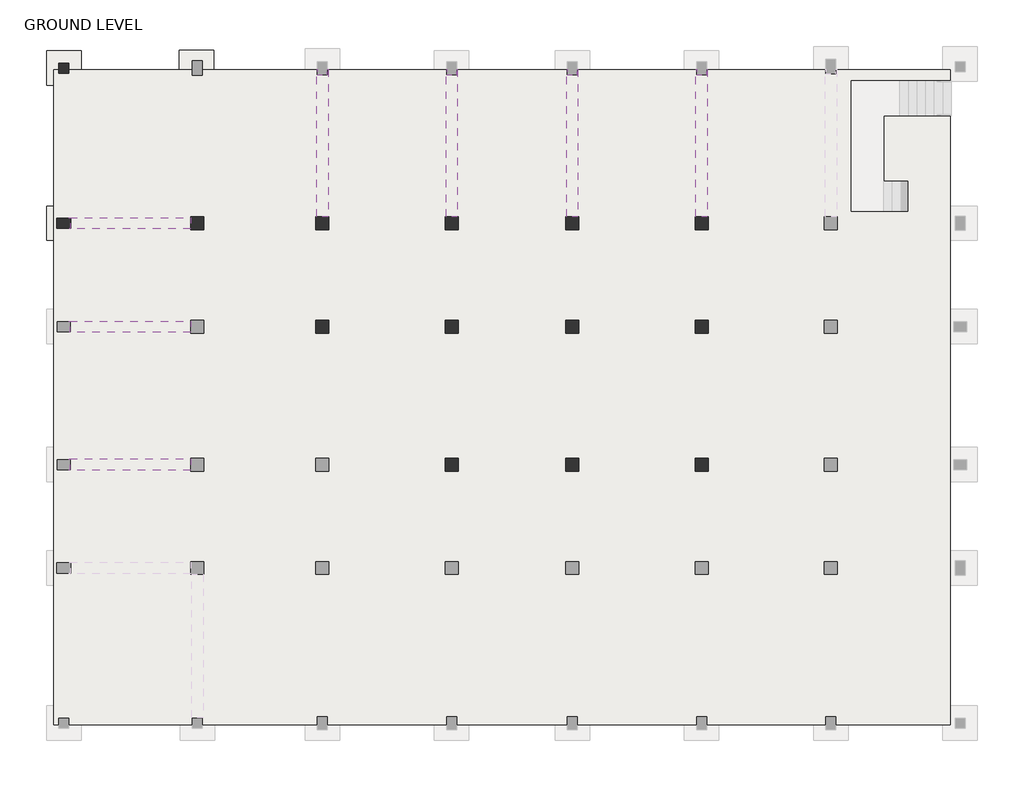
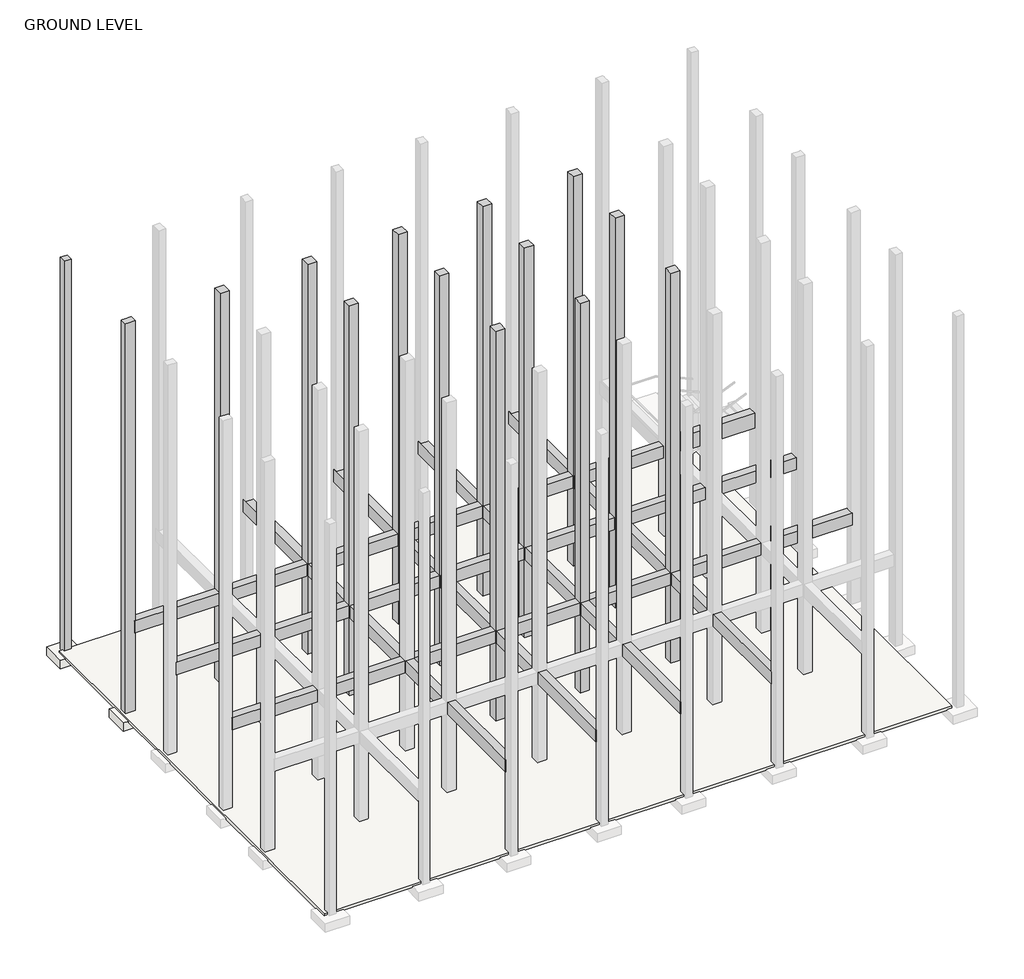
# One storey, part 2 of 3: 16 slabs, 14 columns, 7 beams.
"""IFC4 building model written with IfcOpenShell, lengths in millimetres."""

from ifc_helpers import new_model, si_unit, frame, origin, place, context, project, spatial, polyline, outline, extrude, faceted_brep, element, save

model = new_model("IFC4")

# Units and contexts
model_context = context("Model", 3, world=origin())
ifc_project = project(units=[si_unit("LENGTHUNIT", "METRE", prefix="MILLI")], contexts=[model_context])

# Site, building, storey
site = spatial("IfcSite", under=ifc_project)
building = spatial("IfcBuilding", under=site)
storey = spatial("IfcBuildingStorey", under=building, Name="GROUND LEVEL", Elevation=-1404.4011518)

# Beams
placement = place(None, origin())
element("IfcBeam", 1, ObjectType="M_Concrete-Rectangular Beam : 400 x 800mm", at=placement, inside=storey, context=model_context, shape_type="SweptSolid", body=[
    extrude(outline(polyline([(-16179.7491019, -6019.2309165), (-16535.3491019, -6019.2309165), (-16535.3491019, -6047.8309165), (-16557.5491019, -6047.8309165), (-16557.5491019, -990.0309165), (-16157.5491019, -990.0309165), (-16157.5491019, -6047.8309165), (-16179.7491019, -6047.8309165), (-16179.7491019, -6019.2309165)])), frame((0.0, 0.0, 114.4), z_axis=(0.0, 0.0, 1.0), x_axis=(1.0, 0.0, 0.0)), (0.0, 0.0, 1.0), 647.6),
    extrude(outline(polyline([(-16535.3491019, 16688.3690835), (-16179.7491019, 16688.3690835), (-16179.7491019, 16869.3690835), (-16157.5491019, 16869.3690835), (-16157.5491019, 11659.1690835), (-16557.5491019, 11659.1690835), (-16557.5491019, 16869.3690835), (-16535.3491019, 16869.3690835), (-16535.3491019, 16688.3690835)])), frame((0.0, 0.0, 114.4), z_axis=(0.0, 0.0, 1.0), x_axis=(1.0, 0.0, 0.0)), (0.0, 0.0, 1.0), 647.6),
    extrude(outline(polyline([(-16557.5491019, 11201.9690835), (-16157.5491019, 11201.9690835), (-16157.5491019, 8001.5690835), (-16557.5491019, 8001.5690835), (-16557.5491019, 11201.9690835)])), frame((0.0, 0.0, 114.4), z_axis=(0.0, 0.0, 1.0), x_axis=(1.0, 0.0, 0.0)), (0.0, 0.0, 1.0), 647.6),
    extrude(outline(polyline([(-16557.5491019, 7544.3690835), (-16157.5491019, 7544.3690835), (-16157.5491019, 3124.7690835), (-16557.5491019, 3124.7690835), (-16557.5491019, 7544.3690835)])), frame((0.0, 0.0, 114.4), z_axis=(0.0, 0.0, 1.0), x_axis=(1.0, 0.0, 0.0)), (0.0, 0.0, 1.0), 647.6),
    extrude(outline(polyline([(-16557.5491019, 2667.5690835), (-16157.5491019, 2667.5690835), (-16157.5491019, -532.8309165), (-16557.5491019, -532.8309165), (-16557.5491019, 2667.5690835)])), frame((0.0, 0.0, 114.4), z_axis=(0.0, 0.0, 1.0), x_axis=(1.0, 0.0, 0.0)), (0.0, 0.0, 1.0), 647.6),
])
element("IfcBeam", 2, ObjectType="M_Concrete-Rectangular Beam : 400 x 800mm", at=placement, inside=storey, context=model_context, shape_type="SweptSolid", body=[
    extrude(outline(polyline([(-11607.7491019, -6019.2309165), (-11963.3491019, -6019.2309165), (-11963.3491019, -6047.8309165), (-11985.5491019, -6047.8309165), (-11985.5491019, -990.0309165), (-11585.5491019, -990.0309165), (-11585.5491019, -6047.8309165), (-11607.7491019, -6047.8309165), (-11607.7491019, -6019.2309165)])), frame((0.0, 0.0, 114.4), z_axis=(0.0, 0.0, 1.0), x_axis=(1.0, 0.0, 0.0)), (0.0, 0.0, 1.0), 647.6),
    extrude(outline(polyline([(-11963.3491019, 16688.3690835), (-11607.7491019, 16688.3690835), (-11607.7491019, 16869.3690835), (-11585.5491019, 16869.3690835), (-11585.5491019, 11659.1690835), (-11985.5491019, 11659.1690835), (-11985.5491019, 16869.3690835), (-11963.3491019, 16869.3690835), (-11963.3491019, 16688.3690835)])), frame((0.0, 0.0, 114.4), z_axis=(0.0, 0.0, 1.0), x_axis=(1.0, 0.0, 0.0)), (0.0, 0.0, 1.0), 647.6),
    extrude(outline(polyline([(-11985.5491019, 11201.9690835), (-11585.5491019, 11201.9690835), (-11585.5491019, 8001.5690835), (-11985.5491019, 8001.5690835), (-11985.5491019, 11201.9690835)])), frame((0.0, 0.0, 114.4), z_axis=(0.0, 0.0, 1.0), x_axis=(1.0, 0.0, 0.0)), (0.0, 0.0, 1.0), 647.6),
    extrude(outline(polyline([(-11985.5491019, 7544.3690835), (-11585.5491019, 7544.3690835), (-11585.5491019, 3124.7690835), (-11985.5491019, 3124.7690835), (-11985.5491019, 7544.3690835)])), frame((0.0, 0.0, 114.4), z_axis=(0.0, 0.0, 1.0), x_axis=(1.0, 0.0, 0.0)), (0.0, 0.0, 1.0), 647.6),
    extrude(outline(polyline([(-11585.5491019, -532.8309165), (-11985.5491019, -532.8309165), (-11985.5491019, 2667.5690835), (-11585.5491019, 2667.5690835), (-11585.5491019, -532.8309165)])), frame((0.0, 0.0, 114.4), z_axis=(0.0, 0.0, 1.0), x_axis=(1.0, 0.0, 0.0)), (0.0, 0.0, 1.0), 647.6),
])
element("IfcBeam", 3, ObjectType="M_Concrete-Rectangular Beam : 400 x 800mm", at=placement, inside=storey, context=model_context, shape_type="SweptSolid", body=[
    extrude(outline(polyline([(-7340.5491019, -6019.2309165), (-7696.1491019, -6019.2309165), (-7696.1491019, -6047.8309165), (-7718.3491019, -6047.8309165), (-7718.3491019, -990.0309165), (-7318.3491019, -990.0309165), (-7318.3491019, -6047.8309165), (-7340.5491019, -6047.8309165), (-7340.5491019, -6019.2309165)])), frame((0.0, 0.0, 114.4), z_axis=(0.0, 0.0, 1.0), x_axis=(1.0, 0.0, 0.0)), (0.0, 0.0, 1.0), 647.6),
    extrude(outline(polyline([(-7696.1491019, 16688.3690835), (-7340.5491019, 16688.3690835), (-7340.5491019, 16869.3690835), (-7318.3491019, 16869.3690835), (-7318.3491019, 11659.1690835), (-7718.3491019, 11659.1690835), (-7718.3491019, 16869.3690835), (-7696.1491019, 16869.3690835), (-7696.1491019, 16688.3690835)])), frame((0.0, 0.0, 114.4), z_axis=(0.0, 0.0, 1.0), x_axis=(1.0, 0.0, 0.0)), (0.0, 0.0, 1.0), 647.6),
    extrude(outline(polyline([(-7718.3491019, 7544.3690835), (-7318.3491019, 7544.3690835), (-7318.3491019, 3124.7690835), (-7718.3491019, 3124.7690835), (-7718.3491019, 7544.3690835)])), frame((0.0, 0.0, 114.4), z_axis=(0.0, 0.0, 1.0), x_axis=(1.0, 0.0, 0.0)), (0.0, 0.0, 1.0), 647.6),
    extrude(outline(polyline([(-7318.3491019, 8001.5690835), (-7718.3491019, 8001.5690835), (-7718.3491019, 11201.9690835), (-7318.3491019, 11201.9690835), (-7318.3491019, 8001.5690835)])), frame((0.0, 0.0, 114.4), z_axis=(0.0, 0.0, 1.0), x_axis=(1.0, 0.0, 0.0)), (0.0, 0.0, 1.0), 647.6),
    extrude(outline(polyline([(-7318.3491019, -532.8309165), (-7718.3491019, -532.8309165), (-7718.3491019, 2667.5690835), (-7318.3491019, 2667.5690835), (-7318.3491019, -532.8309165)])), frame((0.0, 0.0, 114.4), z_axis=(0.0, 0.0, 1.0), x_axis=(1.0, 0.0, 0.0)), (0.0, 0.0, 1.0), 647.6),
])
element("IfcBeam", 4, ObjectType="M_Concrete-Rectangular Beam : 400 x 800mm", at=placement, inside=storey, context=model_context, shape_type="SweptSolid", body=[
    extrude(outline(polyline([(-2768.5491019, -6019.2309165), (-3124.1491019, -6019.2309165), (-3124.1491019, -6047.8309165), (-3146.3491019, -6047.8309165), (-3146.3491019, -990.0309165), (-2746.3491019, -990.0309165), (-2746.3491019, -6047.8309165), (-2768.5491019, -6047.8309165), (-2768.5491019, -6019.2309165)])), frame((0.0, 0.0, 114.4), z_axis=(0.0, 0.0, 1.0), x_axis=(1.0, 0.0, 0.0)), (0.0, 0.0, 1.0), 647.6),
    extrude(outline(polyline([(-3124.1491019, 16688.3690835), (-2768.5491019, 16688.3690835), (-2768.5491019, 16869.3690835), (-2746.3491019, 16869.3690835), (-2746.3491019, 11659.1690835), (-3146.3491019, 11659.1690835), (-3146.3491019, 16869.3690835), (-3124.1491019, 16869.3690835), (-3124.1491019, 16688.3690835)])), frame((0.0, 0.0, 114.4), z_axis=(0.0, 0.0, 1.0), x_axis=(1.0, 0.0, 0.0)), (0.0, 0.0, 1.0), 647.6),
    extrude(outline(polyline([(-3146.3491019, 11201.9690835), (-2746.3491019, 11201.9690835), (-2746.3491019, 8001.5690835), (-3146.3491019, 8001.5690835), (-3146.3491019, 11201.9690835)])), frame((0.0, 0.0, 114.4), z_axis=(0.0, 0.0, 1.0), x_axis=(1.0, 0.0, 0.0)), (0.0, 0.0, 1.0), 647.6),
    extrude(outline(polyline([(-3146.3491019, 7544.3690835), (-2746.3491019, 7544.3690835), (-2746.3491019, 3124.7690835), (-3146.3491019, 3124.7690835), (-3146.3491019, 7544.3690835)])), frame((0.0, 0.0, 114.4), z_axis=(0.0, 0.0, 1.0), x_axis=(1.0, 0.0, 0.0)), (0.0, 0.0, 1.0), 647.6),
    extrude(outline(polyline([(-2746.3491019, -532.8309165), (-3146.3491019, -532.8309165), (-3146.3491019, 2667.5690835), (-2746.3491019, 2667.5690835), (-2746.3491019, -532.8309165)])), frame((0.0, 0.0, 114.4), z_axis=(0.0, 0.0, 1.0), x_axis=(1.0, 0.0, 0.0)), (0.0, 0.0, 1.0), 647.6),
])
element("IfcBeam", 5, ObjectType="M_Concrete-Rectangular Beam : 400 x 800mm", at=placement, inside=storey, context=model_context, shape_type="SweptSolid", body=[
    extrude(outline(polyline([(-25247.5491019, 11252.7690835), (-25247.5491019, 11608.3690835), (-25301.5491019, 11608.3690835), (-25301.5491019, 11630.5690835), (-21005.7491019, 11630.5690835), (-21005.7491019, 11230.5690835), (-25301.5491019, 11230.5690835), (-25301.5491019, 11252.7690835), (-25247.5491019, 11252.7690835)])), frame((0.0, 0.0, 114.4), z_axis=(0.0, 0.0, 1.0), x_axis=(1.0, 0.0, 0.0)), (0.0, 0.0, 1.0), 647.6),
    extrude(outline(polyline([(-20548.5491019, 11230.5690835), (-20548.5491019, 11630.5690835), (-16586.1491019, 11630.5690835), (-16586.1491019, 11230.5690835), (-20548.5491019, 11230.5690835)])), frame((0.0, 0.0, 114.4), z_axis=(0.0, 0.0, 1.0), x_axis=(1.0, 0.0, 0.0)), (0.0, 0.0, 1.0), 647.6),
    extrude(outline(polyline([(-16128.9491019, 11230.5690835), (-16128.9491019, 11630.5690835), (-12014.1491019, 11630.5690835), (-12014.1491019, 11230.5690835), (-16128.9491019, 11230.5690835)])), frame((0.0, 0.0, 114.4), z_axis=(0.0, 0.0, 1.0), x_axis=(1.0, 0.0, 0.0)), (0.0, 0.0, 1.0), 647.6),
    extrude(outline(polyline([(-11556.9491019, 11230.5690835), (-11556.9491019, 11630.5690835), (-7746.9491019, 11630.5690835), (-7746.9491019, 11230.5690835), (-11556.9491019, 11230.5690835)])), frame((0.0, 0.0, 114.4), z_axis=(0.0, 0.0, 1.0), x_axis=(1.0, 0.0, 0.0)), (0.0, 0.0, 1.0), 647.6),
    extrude(outline(polyline([(-7289.7491019, 11230.5690835), (-7289.7491019, 11630.5690835), (-3174.9491019, 11630.5690835), (-3174.9491019, 11230.5690835), (-7289.7491019, 11230.5690835)])), frame((0.0, 0.0, 114.4), z_axis=(0.0, 0.0, 1.0), x_axis=(1.0, 0.0, 0.0)), (0.0, 0.0, 1.0), 647.6),
    extrude(outline(polyline([(-2717.7491019, 11230.5690835), (-2717.7491019, 11630.5690835), (1397.0508981, 11630.5690835), (1397.0508981, 11230.5690835), (-2717.7491019, 11230.5690835)])), frame((0.0, 0.0, 114.4), z_axis=(0.0, 0.0, 1.0), x_axis=(1.0, 0.0, 0.0)), (0.0, 0.0, 1.0), 647.6),
    extrude(outline(polyline([(1854.2508981, 11230.5690835), (1854.2508981, 11630.5690835), (5997.6508981, 11630.5690835), (5997.6508981, 11230.5690835), (1854.2508981, 11230.5690835)])), frame((0.0, 0.0, 114.4), z_axis=(0.0, 0.0, 1.0), x_axis=(1.0, 0.0, 0.0)), (0.0, 0.0, 1.0), 800.0),
])
element("IfcBeam", 6, ObjectType="M_Concrete-Rectangular Beam : 400 x 800mm", at=placement, inside=storey, context=model_context, shape_type="SweptSolid", body=[
    extrude(outline(polyline([(-25272.9491019, 2718.3690835), (-25272.9491019, 3073.9690835), (-25301.5491019, 3073.9690835), (-25301.5491019, 3096.1690835), (-21005.7491019, 3096.1690835), (-21005.7491019, 2696.1690835), (-25301.5491019, 2696.1690835), (-25301.5491019, 2718.3690835), (-25272.9491019, 2718.3690835)])), frame((0.0, 0.0, 114.4), z_axis=(0.0, 0.0, 1.0), x_axis=(1.0, 0.0, 0.0)), (0.0, 0.0, 1.0), 647.6),
    extrude(outline(polyline([(5969.0508981, 3073.9690835), (5969.0508981, 2718.3690835), (5997.6508981, 2718.3690835), (5997.6508981, 2696.1690835), (1854.2508981, 2696.1690835), (1854.2508981, 3096.1690835), (5997.6508981, 3096.1690835), (5997.6508981, 3073.9690835), (5969.0508981, 3073.9690835)])), frame((0.0, 0.0, 114.4), z_axis=(0.0, 0.0, 1.0), x_axis=(1.0, 0.0, 0.0)), (0.0, 0.0, 1.0), 647.6),
    extrude(outline(polyline([(-20548.5491019, 2696.1690835), (-20548.5491019, 3096.1690835), (-16586.1491019, 3096.1690835), (-16586.1491019, 2696.1690835), (-20548.5491019, 2696.1690835)])), frame((0.0, 0.0, 114.4), z_axis=(0.0, 0.0, 1.0), x_axis=(1.0, 0.0, 0.0)), (0.0, 0.0, 1.0), 647.6),
    extrude(outline(polyline([(-16128.9491019, 2696.1690835), (-16128.9491019, 3096.1690835), (-12014.1491019, 3096.1690835), (-12014.1491019, 2696.1690835), (-16128.9491019, 2696.1690835)])), frame((0.0, 0.0, 114.4), z_axis=(0.0, 0.0, 1.0), x_axis=(1.0, 0.0, 0.0)), (0.0, 0.0, 1.0), 647.6),
    extrude(outline(polyline([(1397.0508981, 3096.1690835), (1397.0508981, 2696.1690835), (-2717.7491019, 2696.1690835), (-2717.7491019, 3096.1690835), (1397.0508981, 3096.1690835)])), frame((0.0, 0.0, 114.4), z_axis=(0.0, 0.0, 1.0), x_axis=(1.0, 0.0, 0.0)), (0.0, 0.0, 1.0), 647.6),
    extrude(outline(polyline([(-3174.9491019, 3096.1690835), (-3174.9491019, 2696.1690835), (-7289.7491019, 2696.1690835), (-7289.7491019, 3096.1690835), (-3174.9491019, 3096.1690835)])), frame((0.0, 0.0, 114.4), z_axis=(0.0, 0.0, 1.0), x_axis=(1.0, 0.0, 0.0)), (0.0, 0.0, 1.0), 647.6),
    extrude(outline(polyline([(-7746.9491019, 3096.1690835), (-7746.9491019, 2696.1690835), (-11556.9491019, 2696.1690835), (-11556.9491019, 3096.1690835), (-7746.9491019, 3096.1690835)])), frame((0.0, 0.0, 114.4), z_axis=(0.0, 0.0, 1.0), x_axis=(1.0, 0.0, 0.0)), (0.0, 0.0, 1.0), 647.6),
])
element("IfcBeam", 7, ObjectType="M_Concrete-Rectangular Beam : 400 x 800mm", at=placement, inside=storey, context=model_context, shape_type="SweptSolid", body=[
    extrude(outline(polyline([(-25272.9491019, 7595.1690835), (-25272.9491019, 7950.7690835), (-25301.5491019, 7950.7690835), (-25301.5491019, 7972.9690835), (-21005.7491019, 7972.9690835), (-21005.7491019, 7572.9690835), (-25301.5491019, 7572.9690835), (-25301.5491019, 7595.1690835), (-25272.9491019, 7595.1690835)])), frame((0.0, 0.0, 114.4), z_axis=(0.0, 0.0, 1.0), x_axis=(1.0, 0.0, 0.0)), (0.0, 0.0, 1.0), 647.6),
    extrude(outline(polyline([(5969.0508981, 7950.7690835), (5969.0508981, 7595.1690835), (5997.6508981, 7595.1690835), (5997.6508981, 7572.9690835), (1854.2508981, 7572.9690835), (1854.2508981, 7972.9690835), (5997.6508981, 7972.9690835), (5997.6508981, 7950.7690835), (5969.0508981, 7950.7690835)])), frame((0.0, 0.0, 114.4), z_axis=(0.0, 0.0, 1.0), x_axis=(1.0, 0.0, 0.0)), (0.0, 0.0, 1.0), 647.6),
    extrude(outline(polyline([(-7289.7491019, 7572.9690835), (-7289.7491019, 7972.9690835), (-3174.9491019, 7972.9690835), (-3174.9491019, 7572.9690835), (-7289.7491019, 7572.9690835)])), frame((0.0, 0.0, 114.4), z_axis=(0.0, 0.0, 1.0), x_axis=(1.0, 0.0, 0.0)), (0.0, 0.0, 1.0), 647.6),
    extrude(outline(polyline([(-7746.9491019, 7972.9690835), (-7746.9491019, 7572.9690835), (-11556.9491019, 7572.9690835), (-11556.9491019, 7972.9690835), (-7746.9491019, 7972.9690835)])), frame((0.0, 0.0, 114.4), z_axis=(0.0, 0.0, 1.0), x_axis=(1.0, 0.0, 0.0)), (0.0, 0.0, 1.0), 647.6),
    extrude(outline(polyline([(1397.0508981, 7972.9690835), (1397.0508981, 7572.9690835), (-2717.7491019, 7572.9690835), (-2717.7491019, 7972.9690835), (1397.0508981, 7972.9690835)])), frame((0.0, 0.0, 114.4), z_axis=(0.0, 0.0, 1.0), x_axis=(1.0, 0.0, 0.0)), (0.0, 0.0, 1.0), 647.6),
    extrude(outline(polyline([(-12014.1491019, 7972.9690835), (-12014.1491019, 7572.9690835), (-16128.9491019, 7572.9690835), (-16128.9491019, 7972.9690835), (-12014.1491019, 7972.9690835)])), frame((0.0, 0.0, 114.4), z_axis=(0.0, 0.0, 1.0), x_axis=(1.0, 0.0, 0.0)), (0.0, 0.0, 1.0), 647.6),
    extrude(outline(polyline([(-16586.1491019, 7972.9690835), (-16586.1491019, 7572.9690835), (-20548.5491019, 7572.9690835), (-20548.5491019, 7972.9690835), (-16586.1491019, 7972.9690835)])), frame((0.0, 0.0, 114.4), z_axis=(0.0, 0.0, 1.0), x_axis=(1.0, 0.0, 0.0)), (0.0, 0.0, 1.0), 647.6),
])

# Columns
element("IfcColumn", 8, ObjectType="M_Concrete-Rectangular-Column : C1", at=placement, inside=storey, context=model_context, shape_type="SweptSolid", body=[
    extrude(outline(polyline([(-25323.7491019, 17094.7690835), (-25323.7491019, 16739.1690835), (-25679.3491019, 16739.1690835), (-25679.3491019, 17094.7690835), (-25323.7491019, 17094.7690835)])), frame((0.0, 0.0, -4147.6011518), z_axis=(0.0, 0.0, 1.0), x_axis=(1.0, 0.0, 0.0)), (0.0, 0.0, 1.0), 20911.6011518),
])
element("IfcColumn", 9, ObjectType="M_Concrete-Rectangular-Column : C3", at=placement, inside=storey, context=model_context, shape_type="SweptSolid", body=[
    extrude(outline(polyline([(-7289.7491019, 8001.5690835), (-7289.7491019, 7544.3690835), (-7746.9491019, 7544.3690835), (-7746.9491019, 8001.5690835), (-7289.7491019, 8001.5690835)])), frame((0.0, 0.0, -4147.6011518), z_axis=(0.0, 0.0, 1.0), x_axis=(1.0, 0.0, 0.0)), (0.0, 0.0, 1.0), 20911.6011518),
])
element("IfcColumn", 10, ObjectType="M_Concrete-Rectangular-Column : C3", at=placement, inside=storey, context=model_context, shape_type="SweptSolid", body=[
    extrude(outline(polyline([(-20548.5491019, 11659.1690835), (-20548.5491019, 11201.9690835), (-21005.7491019, 11201.9690835), (-21005.7491019, 11659.1690835), (-20548.5491019, 11659.1690835)])), frame((0.0, 0.0, -4147.6011518), z_axis=(0.0, 0.0, 1.0), x_axis=(1.0, 0.0, 0.0)), (0.0, 0.0, 1.0), 20911.6011518),
])
element("IfcColumn", 11, ObjectType="M_Concrete-Rectangular-Column : C3", at=placement, inside=storey, context=model_context, shape_type="SweptSolid", body=[
    extrude(outline(polyline([(-16128.9491019, 11659.1690835), (-16128.9491019, 11201.9690835), (-16586.1491019, 11201.9690835), (-16586.1491019, 11659.1690835), (-16128.9491019, 11659.1690835)])), frame((0.0, 0.0, -4147.6011518), z_axis=(0.0, 0.0, 1.0), x_axis=(1.0, 0.0, 0.0)), (0.0, 0.0, 1.0), 20911.6011518),
])
element("IfcColumn", 12, ObjectType="M_Concrete-Rectangular-Column : C3", at=placement, inside=storey, context=model_context, shape_type="SweptSolid", body=[
    extrude(outline(polyline([(-11556.9491019, 11659.1690835), (-11556.9491019, 11201.9690835), (-12014.1491019, 11201.9690835), (-12014.1491019, 11659.1690835), (-11556.9491019, 11659.1690835)])), frame((0.0, 0.0, -4147.6011518), z_axis=(0.0, 0.0, 1.0), x_axis=(1.0, 0.0, 0.0)), (0.0, 0.0, 1.0), 20911.6011518),
])
element("IfcColumn", 13, ObjectType="M_Concrete-Rectangular-Column : C3", at=placement, inside=storey, context=model_context, shape_type="SweptSolid", body=[
    extrude(outline(polyline([(-7289.7491019, 11659.1690835), (-7289.7491019, 11201.9690835), (-7746.9491019, 11201.9690835), (-7746.9491019, 11659.1690835), (-7289.7491019, 11659.1690835)])), frame((0.0, 0.0, -4147.6011518), z_axis=(0.0, 0.0, 1.0), x_axis=(1.0, 0.0, 0.0)), (0.0, 0.0, 1.0), 20911.6011518),
])
element("IfcColumn", 14, ObjectType="M_Concrete-Rectangular-Column : C3", at=placement, inside=storey, context=model_context, shape_type="SweptSolid", body=[
    extrude(outline(polyline([(-2717.7491019, 11659.1690835), (-2717.7491019, 11201.9690835), (-3174.9491019, 11201.9690835), (-3174.9491019, 11659.1690835), (-2717.7491019, 11659.1690835)])), frame((0.0, 0.0, -4147.6011518), z_axis=(0.0, 0.0, 1.0), x_axis=(1.0, 0.0, 0.0)), (0.0, 0.0, 1.0), 20911.6011518),
])
element("IfcColumn", 15, ObjectType="M_Concrete-Rectangular-Column : C3", at=placement, inside=storey, context=model_context, shape_type="SweptSolid", body=[
    extrude(outline(polyline([(-2717.7491019, 8001.5690835), (-2717.7491019, 7544.3690835), (-3174.9491019, 7544.3690835), (-3174.9491019, 8001.5690835), (-2717.7491019, 8001.5690835)])), frame((0.0, 0.0, -4147.6011518), z_axis=(0.0, 0.0, 1.0), x_axis=(1.0, 0.0, 0.0)), (0.0, 0.0, 1.0), 20911.6011518),
])
element("IfcColumn", 16, ObjectType="M_Concrete-Rectangular-Column : C3", at=placement, inside=storey, context=model_context, shape_type="SweptSolid", body=[
    extrude(outline(polyline([(-11556.9491019, 8001.5690835), (-11556.9491019, 7544.3690835), (-12014.1491019, 7544.3690835), (-12014.1491019, 8001.5690835), (-11556.9491019, 8001.5690835)])), frame((0.0, 0.0, -4147.6011518), z_axis=(0.0, 0.0, 1.0), x_axis=(1.0, 0.0, 0.0)), (0.0, 0.0, 1.0), 20911.6011518),
])
element("IfcColumn", 17, ObjectType="M_Concrete-Rectangular-Column : C3", at=placement, inside=storey, context=model_context, shape_type="SweptSolid", body=[
    extrude(outline(polyline([(-16128.9491019, 8001.5690835), (-16128.9491019, 7544.3690835), (-16586.1491019, 7544.3690835), (-16586.1491019, 8001.5690835), (-16128.9491019, 8001.5690835)])), frame((0.0, 0.0, -4147.6011518), z_axis=(0.0, 0.0, 1.0), x_axis=(1.0, 0.0, 0.0)), (0.0, 0.0, 1.0), 20911.6011518),
])
element("IfcColumn", 18, ObjectType="M_Concrete-Rectangular-Column : C3", at=placement, inside=storey, context=model_context, shape_type="SweptSolid", body=[
    extrude(outline(polyline([(-2717.7491019, 3124.7690835), (-2717.7491019, 2667.5690835), (-3174.9491019, 2667.5690835), (-3174.9491019, 3124.7690835), (-2717.7491019, 3124.7690835)])), frame((0.0, 0.0, -4147.6011518), z_axis=(0.0, 0.0, 1.0), x_axis=(1.0, 0.0, 0.0)), (0.0, 0.0, 1.0), 20911.6011518),
])
element("IfcColumn", 19, ObjectType="M_Concrete-Rectangular-Column : C3", at=placement, inside=storey, context=model_context, shape_type="SweptSolid", body=[
    extrude(outline(polyline([(-7289.7491019, 3124.7690835), (-7289.7491019, 2667.5690835), (-7746.9491019, 2667.5690835), (-7746.9491019, 3124.7690835), (-7289.7491019, 3124.7690835)])), frame((0.0, 0.0, -4147.6011518), z_axis=(0.0, 0.0, 1.0), x_axis=(1.0, 0.0, 0.0)), (0.0, 0.0, 1.0), 20911.6011518),
])
element("IfcColumn", 20, ObjectType="M_Concrete-Rectangular-Column : C3", at=placement, inside=storey, context=model_context, shape_type="SweptSolid", body=[
    extrude(outline(polyline([(-11556.9491019, 3124.7690835), (-11556.9491019, 2667.5690835), (-12014.1491019, 2667.5690835), (-12014.1491019, 3124.7690835), (-11556.9491019, 3124.7690835)])), frame((0.0, 0.0, -4147.6011518), z_axis=(0.0, 0.0, 1.0), x_axis=(1.0, 0.0, 0.0)), (0.0, 0.0, 1.0), 20911.6011518),
])
element("IfcColumn", 21, ObjectType="M_Concrete-Rectangular-Column : C4", at=placement, inside=storey, context=model_context, shape_type="Brep", body=[
    faceted_brep([(-25755.5491019, 11608.3690835, -4147.6011518), (-25247.5491019, 11608.3690835, -4147.6011518), (-25247.5491019, 11252.7690835, -4147.6011518), (-25755.5491019, 11252.7690835, -4147.6011518), (-25755.5491019, 11608.3690835, 16764.0), (-25701.5491019, 11608.3690835, 16764.0), (-25679.3491019, 11608.3690835, 16764.0), (-25247.5491019, 11608.3690835, 16764.0), (-25247.5491019, 11252.7690835, 16764.0), (-25679.3491019, 11252.7690835, 16764.0), (-25701.5491019, 11252.7690835, 16764.0), (-25755.5491019, 11252.7690835, 16764.0)], [[[0, 1, 2, 3]], [[4, 5, 6, 7, 1, 0]], [[7, 8, 2, 1]], [[8, 9, 10, 11, 3, 2]], [[11, 4, 0, 3]], [[4, 11, 10, 9, 8, 7, 6, 5]]]),
])

# Slabs
element("IfcSlab", 22, ObjectType="6\" Foundation Slab", at=placement, inside=storey, context=model_context, shape_type="Brep", body=[
    faceted_brep([(5842.0508981, 16861.9544764, -4197.8282159), (5842.0508981, 16459.7690835, -4197.8282159), (5842.0508981, 12040.1690835, -4197.8282159), (5842.0508981, 10820.9690835, -4197.8282159), (5842.0508981, 8382.5690835, -4197.8282159), (5842.0508981, 7163.3690835, -4197.8282159), (5842.0508981, 3505.7690835, -4197.8282159), (5842.0508981, 2286.5690835, -4197.8282159), (5842.0508981, -151.8309165, -4197.8282159), (5842.0508981, -1371.0309165, -4197.8282159), (5842.0508981, -5638.2309165, -4197.8282159), (5842.0508981, -6302.8455236, -4197.8282159), (5588.0508981, -6302.8455236, -4197.8282159), (2235.2508981, -6302.8455236, -4197.8282159), (1016.0508981, -6302.8455236, -4197.8282159), (-2336.7491019, -6302.8455236, -4197.8282159), (-3555.9491019, -6302.8455236, -4197.8282159), (-6908.7491019, -6302.8455236, -4197.8282159), (-8127.9491019, -6302.8455236, -4197.8282159), (-11175.9491019, -6302.8455236, -4197.8282159), (-12395.1491019, -6302.8455236, -4197.8282159), (-15747.9491019, -6302.8455236, -4197.8282159), (-16967.1491019, -6302.8455236, -4197.8282159), (-20167.5491019, -6302.8455236, -4197.8282159), (-21386.7491019, -6302.8455236, -4197.8282159), (-24891.9491019, -6302.8455236, -4197.8282159), (-25857.1491019, -6302.8455236, -4197.8282159), (-25857.1491019, -5638.2309165, -4197.8282159), (-25857.1491019, -1371.0309165, -4197.8282159), (-25857.1491019, -151.8309165, -4197.8282159), (-25857.1491019, 2286.5690835, -4197.8282159), (-25857.1491019, 3505.7690835, -4197.8282159), (-25857.1491019, 7163.3690835, -4197.8282159), (-25857.1491019, 8382.5690835, -4197.8282159), (-25857.1491019, 10820.9690835, -4197.8282159), (-25857.1491019, 12040.1690835, -4197.8282159), (-25857.1491019, 16307.3690835, -4197.8282159), (-25857.1491019, 16861.9544764, -4197.8282159), (-24891.9491019, 16861.9544764, -4197.8282159), (-21412.1491019, 16861.9544764, -4197.8282159), (-20192.9491019, 16861.9544764, -4197.8282159), (-16967.1491019, 16861.9544764, -4197.8282159), (-15747.9491019, 16861.9544764, -4197.8282159), (-12395.1491019, 16861.9544764, -4197.8282159), (-11175.9491019, 16861.9544764, -4197.8282159), (-8127.9491019, 16861.9544764, -4197.8282159), (-6908.7491019, 16861.9544764, -4197.8282159), (-3555.9491019, 16861.9544764, -4197.8282159), (-2336.7491019, 16861.9544764, -4197.8282159), (1016.0508981, 16861.9544764, -4197.8282159), (2235.2508981, 16861.9544764, -4197.8282159), (5588.0508981, 16861.9544764, -4197.8282159), (5842.0508981, 16861.9544764, -4045.4282159), (-25857.1491019, 16861.9544764, -4045.4282159), (-25857.1491019, -6302.8455236, -4045.4282159), (5842.0508981, -6302.8455236, -4045.4282159), (5842.0508981, 16861.9544764, -4147.6011518), (5842.0508981, -6302.8455236, -4147.6011518), (-25857.1491019, -6302.8455236, -4147.6011518), (-25857.1491019, 16861.9544764, -4147.6011518)], [[[0, 1, 2, 3, 4, 5, 6, 7, 8, 9, 10, 11, 12, 13, 14, 15, 16, 17, 18, 19, 20, 21, 22, 23, 24, 25, 26, 27, 28, 29, 30, 31, 32, 33, 34, 35, 36, 37, 38, 39, 40, 41, 42, 43, 44, 45, 46, 47, 48, 49, 50, 51]], [[52, 53, 54, 55]], [[11, 10, 9, 8, 7, 6, 5, 4, 3, 2, 1, 0, 56, 52, 55, 57]], [[26, 25, 24, 23, 22, 21, 20, 19, 18, 17, 16, 15, 14, 13, 12, 11, 57, 55, 54, 58]], [[37, 36, 35, 34, 33, 32, 31, 30, 29, 28, 27, 26, 58, 54, 53, 59]], [[0, 51, 50, 49, 48, 47, 46, 45, 44, 43, 42, 41, 40, 39, 38, 37, 59, 53, 52, 56]]]),
])
element("IfcSlab", 23, ObjectType="M_Footing-Rectangular : F 5", at=placement, inside=storey, context=model_context, shape_type="Brep", body=[
    faceted_brep([(-24891.9491019, 17526.5690835, -4147.6011518), (-26111.1491019, 17526.5690835, -4147.6011518), (-26111.1491019, 16307.3690835, -4147.6011518), (-25857.1491019, 16307.3690835, -4147.6011518), (-25857.1491019, 16861.9544764, -4147.6011518), (-24891.9491019, 16861.9544764, -4147.6011518), (-24891.9491019, 17526.5690835, -4597.6011518), (-24891.9491019, 16307.3690835, -4597.6011518), (-26111.1491019, 16307.3690835, -4597.6011518), (-26111.1491019, 17526.5690835, -4597.6011518), (-24891.9491019, 16307.3690835, -4197.8282159), (-25857.1491019, 16307.3690835, -4197.8282159), (-24891.9491019, 16861.9544764, -4197.8282159), (-25857.1491019, 16861.9544764, -4197.8282159)], [[[0, 1, 2, 3, 4, 5]], [[6, 7, 8, 9]], [[1, 0, 6, 9]], [[2, 1, 9, 8]], [[8, 7, 10, 11, 3, 2]], [[7, 6, 0, 5, 12, 10]], [[12, 13, 11, 10]], [[13, 12, 5, 4]], [[11, 13, 4, 3]]]),
])
element("IfcSlab", 24, ObjectType="M_Footing-Rectangular : F 5", at=placement, inside=storey, context=model_context, shape_type="SweptSolid", body=[
    extrude(outline(polyline([(17551.9690835, -4597.6011518), (16332.7690835, -4597.6011518), (16332.7690835, -4197.8282159), (16861.9544764, -4197.8282159), (16861.9544764, -4147.6011518), (17551.9690835, -4147.6011518), (17551.9690835, -4597.6011518)])), frame((-21412.1491019, 0.0, 0.0), z_axis=(1.0, 0.0, 0.0), x_axis=(0.0, 1.0, 0.0)), (0.0, 0.0, 1.0), 1219.2),
])
element("IfcSlab", 25, ObjectType="M_Footing-Rectangular : F 5", at=placement, inside=storey, context=model_context, shape_type="SweptSolid", body=[
    extrude(outline(polyline([(-2336.7491019, 12040.1690835), (-2336.7491019, 10820.9690835), (-3555.9491019, 10820.9690835), (-3555.9491019, 12040.1690835), (-2336.7491019, 12040.1690835)])), frame((0.0, 0.0, -4597.6011518), z_axis=(0.0, 0.0, 1.0), x_axis=(1.0, 0.0, 0.0)), (0.0, 0.0, 1.0), 399.772936),
])
element("IfcSlab", 26, ObjectType="M_Footing-Rectangular : F 5", at=placement, inside=storey, context=model_context, shape_type="SweptSolid", body=[
    extrude(outline(polyline([(-6908.7491019, 12040.1690835), (-6908.7491019, 10820.9690835), (-8127.9491019, 10820.9690835), (-8127.9491019, 12040.1690835), (-6908.7491019, 12040.1690835)])), frame((0.0, 0.0, -4597.6011518), z_axis=(0.0, 0.0, 1.0), x_axis=(1.0, 0.0, 0.0)), (0.0, 0.0, 1.0), 399.772936),
])
element("IfcSlab", 27, ObjectType="M_Footing-Rectangular : F 5", at=placement, inside=storey, context=model_context, shape_type="SweptSolid", body=[
    extrude(outline(polyline([(-11175.9491019, 12040.1690835), (-11175.9491019, 10820.9690835), (-12395.1491019, 10820.9690835), (-12395.1491019, 12040.1690835), (-11175.9491019, 12040.1690835)])), frame((0.0, 0.0, -4597.6011518), z_axis=(0.0, 0.0, 1.0), x_axis=(1.0, 0.0, 0.0)), (0.0, 0.0, 1.0), 399.772936),
])
element("IfcSlab", 28, ObjectType="M_Footing-Rectangular : F 5", at=placement, inside=storey, context=model_context, shape_type="SweptSolid", body=[
    extrude(outline(polyline([(-15747.9491019, 12040.1690835), (-15747.9491019, 10820.9690835), (-16967.1491019, 10820.9690835), (-16967.1491019, 12040.1690835), (-15747.9491019, 12040.1690835)])), frame((0.0, 0.0, -4597.6011518), z_axis=(0.0, 0.0, 1.0), x_axis=(1.0, 0.0, 0.0)), (0.0, 0.0, 1.0), 399.772936),
])
element("IfcSlab", 29, ObjectType="M_Footing-Rectangular : F 5", at=placement, inside=storey, context=model_context, shape_type="SweptSolid", body=[
    extrude(outline(polyline([(-20167.5491019, 12040.1690835), (-20167.5491019, 10820.9690835), (-21386.7491019, 10820.9690835), (-21386.7491019, 12040.1690835), (-20167.5491019, 12040.1690835)])), frame((0.0, 0.0, -4597.6011518), z_axis=(0.0, 0.0, 1.0), x_axis=(1.0, 0.0, 0.0)), (0.0, 0.0, 1.0), 399.772936),
])
element("IfcSlab", 30, ObjectType="M_Footing-Rectangular : F 5", at=placement, inside=storey, context=model_context, shape_type="SweptSolid", body=[
    extrude(outline(polyline([(-4597.6011518, -26111.1491019), (-4597.6011518, -24891.9491019), (-4197.8282159, -24891.9491019), (-4197.8282159, -25857.1491019), (-4147.6011518, -25857.1491019), (-4147.6011518, -26111.1491019), (-4597.6011518, -26111.1491019)])), frame((0.0, 10820.9690835, 0.0), z_axis=(0.0, 1.0, 0.0), x_axis=(0.0, 0.0, 1.0)), (0.0, 0.0, 1.0), 1219.2),
])
element("IfcSlab", 31, ObjectType="M_Footing-Rectangular : F 5", at=placement, inside=storey, context=model_context, shape_type="SweptSolid", body=[
    extrude(outline(polyline([(-15747.9491019, 8382.5690835), (-15747.9491019, 7163.3690835), (-16967.1491019, 7163.3690835), (-16967.1491019, 8382.5690835), (-15747.9491019, 8382.5690835)])), frame((0.0, 0.0, -4597.6011518), z_axis=(0.0, 0.0, 1.0), x_axis=(1.0, 0.0, 0.0)), (0.0, 0.0, 1.0), 399.772936),
])
element("IfcSlab", 32, ObjectType="M_Footing-Rectangular : F 5", at=placement, inside=storey, context=model_context, shape_type="SweptSolid", body=[
    extrude(outline(polyline([(-11175.9491019, 8382.5690835), (-11175.9491019, 7163.3690835), (-12395.1491019, 7163.3690835), (-12395.1491019, 8382.5690835), (-11175.9491019, 8382.5690835)])), frame((0.0, 0.0, -4597.6011518), z_axis=(0.0, 0.0, 1.0), x_axis=(1.0, 0.0, 0.0)), (0.0, 0.0, 1.0), 399.772936),
])
element("IfcSlab", 33, ObjectType="M_Footing-Rectangular : F 5", at=placement, inside=storey, context=model_context, shape_type="SweptSolid", body=[
    extrude(outline(polyline([(-6908.7491019, 8382.5690835), (-6908.7491019, 7163.3690835), (-8127.9491019, 7163.3690835), (-8127.9491019, 8382.5690835), (-6908.7491019, 8382.5690835)])), frame((0.0, 0.0, -4597.6011518), z_axis=(0.0, 0.0, 1.0), x_axis=(1.0, 0.0, 0.0)), (0.0, 0.0, 1.0), 399.772936),
])
element("IfcSlab", 34, ObjectType="M_Footing-Rectangular : F 5", at=placement, inside=storey, context=model_context, shape_type="SweptSolid", body=[
    extrude(outline(polyline([(-2336.7491019, 8382.5690835), (-2336.7491019, 7163.3690835), (-3555.9491019, 7163.3690835), (-3555.9491019, 8382.5690835), (-2336.7491019, 8382.5690835)])), frame((0.0, 0.0, -4597.6011518), z_axis=(0.0, 0.0, 1.0), x_axis=(1.0, 0.0, 0.0)), (0.0, 0.0, 1.0), 399.772936),
])
element("IfcSlab", 35, ObjectType="M_Footing-Rectangular : F 5", at=placement, inside=storey, context=model_context, shape_type="SweptSolid", body=[
    extrude(outline(polyline([(-2336.7491019, 3505.7690835), (-2336.7491019, 2286.5690835), (-3555.9491019, 2286.5690835), (-3555.9491019, 3505.7690835), (-2336.7491019, 3505.7690835)])), frame((0.0, 0.0, -4597.6011518), z_axis=(0.0, 0.0, 1.0), x_axis=(1.0, 0.0, 0.0)), (0.0, 0.0, 1.0), 399.772936),
])
element("IfcSlab", 36, ObjectType="M_Footing-Rectangular : F 5", at=placement, inside=storey, context=model_context, shape_type="SweptSolid", body=[
    extrude(outline(polyline([(-6908.7491019, 3505.7690835), (-6908.7491019, 2286.5690835), (-8127.9491019, 2286.5690835), (-8127.9491019, 3505.7690835), (-6908.7491019, 3505.7690835)])), frame((0.0, 0.0, -4597.6011518), z_axis=(0.0, 0.0, 1.0), x_axis=(1.0, 0.0, 0.0)), (0.0, 0.0, 1.0), 399.772936),
])
element("IfcSlab", 37, ObjectType="M_Footing-Rectangular : F 5", at=placement, inside=storey, context=model_context, shape_type="SweptSolid", body=[
    extrude(outline(polyline([(-11175.9491019, 3505.7690835), (-11175.9491019, 2286.5690835), (-12395.1491019, 2286.5690835), (-12395.1491019, 3505.7690835), (-11175.9491019, 3505.7690835)])), frame((0.0, 0.0, -4597.6011518), z_axis=(0.0, 0.0, 1.0), x_axis=(1.0, 0.0, 0.0)), (0.0, 0.0, 1.0), 399.772936),
])

save(model, "model.ifc")

# Revit data of these elements
# Type "M_Concrete-Rectangular Beam : 400 x 800mm"
#   Length [instance default] = 5' - 0"
#   b = 1' - 3.74803"
#   h = 2' - 7.49606"
#   Structural Material [instance default] = Concrete, Cast-in-Place gray
#   Assembly Code = ""
# Type "M_Concrete-Rectangular-Column : C1"
#   b = 1' - 2"
#   h = 1' - 2"
#   Structural Material [instance default] = Concrete, Cast-in-Place gray
# Type "M_Concrete-Rectangular-Column : C3"
#   b = 1' - 6"
#   h = 1' - 6"
#   Structural Material [instance default] = Concrete, Cast-in-Place gray
# Type "M_Concrete-Rectangular-Column : C4"
#   b = 1' - 2"
#   h = 1' - 8"
#   Structural Material [instance default] = Concrete, Cast-in-Place gray
# Type "6\" Foundation Slab"
#   Layers, outside or top first: 0' - 6" "Concrete, Cast-in-Place gray" (function 1)
# Type "M_Footing-Rectangular : F 5"
#   Width = 4' - 0"
#   Length = 4' - 0"
#   Thickness = 1' - 5.71654"
#   Structural Material [instance default] = Concrete, Cast-in-Place gray
#   Assembly Code = ""
# Elements 1, 2, 3, 4, 5, 6, 7 (IfcBeam, "M_Concrete-Rectangular Beam : 400 x 800mm")
#   Comments = ""
#   Structural Material = Concrete, Cast-in-Place gray
#   Phase Created = New Construction
#   Materials on its faces: "Concrete, Cast-in-Place gray"
# Element 8 (IfcColumn, "M_Concrete-Rectangular-Column : C1")
#   Comments = ""
#   Structural Material = Concrete, Cast-in-Place gray
#   Phase Created = New Construction
#   Materials on its faces: "Concrete, Cast-in-Place gray"
# Elements 9, 10, 11, 12, 13, 14, 15, 16, 17, 18, 19, 20 (IfcColumn, "M_Concrete-Rectangular-Column : C3")
#   Comments = ""
#   Structural Material = Concrete, Cast-in-Place gray
#   Phase Created = New Construction
#   Materials on its faces: "Concrete, Cast-in-Place gray"
# Element 21 (IfcColumn, "M_Concrete-Rectangular-Column : C4")
#   Comments = ""
#   Structural Material = Concrete, Cast-in-Place gray
#   Phase Created = New Construction
#   Materials on its faces: "Concrete, Cast-in-Place gray"
# Element 22 (IfcSlab, "6\" Foundation Slab")
#   Height Offset From Level = -8' - 7.97744"
#   built-in parameter 1001954 = 1
#   Phase Created = New Construction
#   Materials on its faces: "Concrete, Cast-in-Place gray"
# Elements 23, 24, 25, 26, 27, 28, 29, 30, 31, 32, 33, 34, 35, 36, 37 (IfcSlab, "M_Footing-Rectangular : F 5")
#   Comments = ""
#   Structural Material = Concrete, Cast-in-Place gray
#   Phase Created = New Construction
#   Materials on its faces: "Concrete, Cast-in-Place gray"
# Materials
#   "Concrete, Cast-in-Place gray": class "Concrete", colour RGB 192 192 192, transparency 0, Description = "Cast-in-place concrete", Cost = 0
